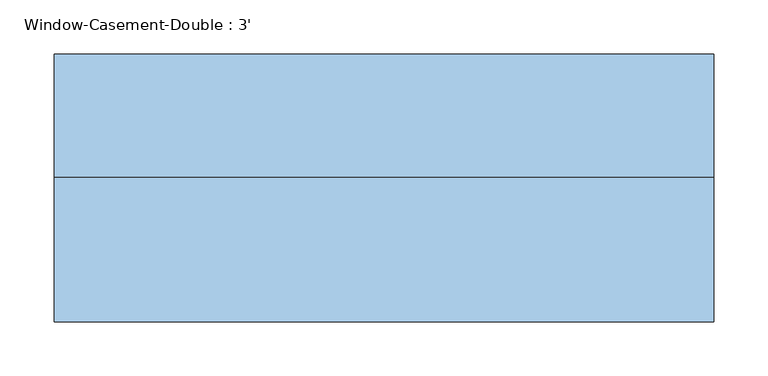
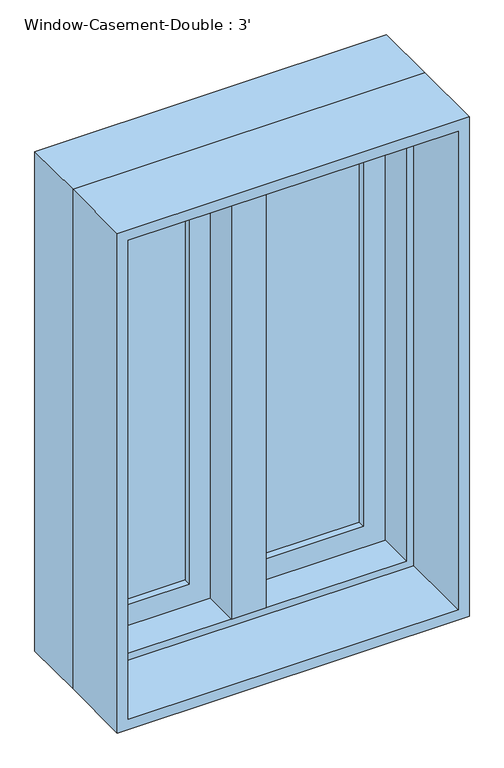
"""IFC4 building model written with IfcOpenShell, lengths in millimetres: window geometry, Window-Casement-Double : 3'."""

from ifc_helpers import new_model, si_unit, frame, origin, place, context, project, spatial, polyline, outline, extrude, faceted_brep, source, transform, mapped, element, save


def window_casement_double_3_c417fced(model_context):
    return source(origin(), model_context, "Body", "SolidModel", [
        faceted_brep([(9.525, 133.35, 1816.1), (-9.525, 133.35, 1816.1), (-9.525, 82.55, 1816.1), (9.525, 82.55, 1816.1), (9.525, 133.35, 927.1), (9.525, 82.55, 927.1), (-9.525, 82.55, 927.1), (-9.525, 133.35, 927.1), (-9.525, 82.55, 946.15), (-9.525, 82.55, 1797.05), (-30.1625, 82.55, 946.15), (-30.1625, 82.55, 1797.05), (-30.1625, 19.05, 946.15), (-30.1625, 19.05, 1797.05), (30.1625, 19.05, 946.15), (30.1625, 19.05, 1797.05), (30.1625, 82.55, 946.15), (30.1625, 82.55, 1797.05), (9.525, 82.55, 946.15), (9.525, 82.55, 1797.05)], [[[0, 1, 2, 3]], [[4, 5, 6, 7]], [[1, 0, 4, 7]], [[2, 1, 7, 6, 8, 9]], [[9, 8, 10, 11]], [[11, 10, 12, 13]], [[13, 12, 14, 15]], [[15, 14, 16, 17]], [[17, 16, 18, 19]], [[0, 3, 19, 18, 5, 4]], [[18, 8, 6, 5]], [[9, 19, 3, 2]], [[8, 18, 16, 14, 12, 10]], [[19, 9, 11, 13, 15, 17]]]),
        extrude(outline(polyline([(-66.675, 114.3), (-66.675, 107.95), (-234.95, 107.95), (-234.95, 114.3), (-66.675, 114.3)])), frame((0.0, 0.0, 984.25), z_axis=(0.0, 0.0, 1.0), x_axis=(1.0, 0.0, 0.0)), (0.0, 0.0, 1.0), 774.7),
        extrude(outline(polyline([(-234.95, 95.25), (-234.95, 101.6), (-66.675, 101.6), (-66.675, 95.25), (-234.95, 95.25)])), frame((0.0, 0.0, 984.25), z_axis=(0.0, 0.0, 1.0), x_axis=(1.0, 0.0, 0.0)), (0.0, 0.0, 1.0), 774.7),
        extrude(outline(polyline([(234.95, 114.3), (234.95, 107.95), (66.675, 107.95), (66.675, 114.3), (234.95, 114.3)])), frame((0.0, 0.0, 984.25), z_axis=(0.0, 0.0, 1.0), x_axis=(1.0, 0.0, 0.0)), (0.0, 0.0, 1.0), 774.7),
        extrude(outline(polyline([(66.675, 95.25), (66.675, 101.6), (234.95, 101.6), (234.95, 95.25), (66.675, 95.25)])), frame((0.0, 0.0, 984.25), z_axis=(0.0, 0.0, 1.0), x_axis=(1.0, 0.0, 0.0)), (0.0, 0.0, 1.0), 774.7),
        extrude(outline(polyline([(1816.1, -292.1), (927.1, -292.1), (927.1, -9.525), (1816.1, -9.525), (1816.1, -292.1)]), holes=[polyline([(1758.95, -66.675), (984.25, -66.675), (984.25, -234.95), (1758.95, -234.95), (1758.95, -66.675)])]), frame((0.0, 82.55, 0.0), z_axis=(0.0, 1.0, 0.0), x_axis=(0.0, 0.0, 1.0)), (0.0, 0.0, 1.0), 44.45),
        extrude(outline(polyline([(927.1, 292.1), (1816.1, 292.1), (1816.1, 9.525), (927.1, 9.525), (927.1, 292.1)]), holes=[polyline([(984.25, 66.675), (1758.95, 66.675), (1758.95, 234.95), (984.25, 234.95), (984.25, 66.675)])]), frame((0.0, 82.55, 0.0), z_axis=(0.0, 1.0, 0.0), x_axis=(0.0, 0.0, 1.0)), (0.0, 0.0, 1.0), 44.45),
        extrude(outline(polyline([(1828.8, -304.8), (914.4, -304.8), (914.4, 304.8), (1828.8, 304.8), (1828.8, -304.8)]), holes=[polyline([(1809.75, 285.75), (933.45, 285.75), (933.45, -285.75), (1809.75, -285.75), (1809.75, 285.75)])]), frame((0.0, -114.3, 0.0), z_axis=(0.0, 1.0, 0.0), x_axis=(0.0, 0.0, 1.0)), (0.0, 0.0, 1.0), 133.35),
        faceted_brep([(273.05, 82.55, 1797.05), (273.05, 19.05, 1797.05), (-273.05, 19.05, 1797.05), (-273.05, 82.55, 1797.05), (292.1, 133.35, 1816.1), (292.1, 82.55, 1816.1), (-292.1, 82.55, 1816.1), (-292.1, 133.35, 1816.1), (304.8, 19.05, 1828.8), (304.8, 133.35, 1828.8), (-304.8, 133.35, 1828.8), (-304.8, 19.05, 1828.8), (-273.05, 19.05, 946.15), (-273.05, 82.55, 946.15), (-292.1, 82.55, 927.1), (-292.1, 133.35, 927.1), (-304.8, 133.35, 914.4), (-304.8, 19.05, 914.4), (273.05, 19.05, 946.15), (273.05, 82.55, 946.15), (292.1, 82.55, 927.1), (292.1, 133.35, 927.1), (304.8, 133.35, 914.4), (304.8, 19.05, 914.4)], [[[0, 1, 2, 3]], [[4, 5, 6, 7]], [[8, 9, 10, 11]], [[3, 2, 12, 13]], [[7, 6, 14, 15]], [[11, 10, 16, 17]], [[13, 12, 18, 19]], [[15, 14, 20, 21]], [[17, 16, 22, 23]], [[11, 17, 23, 8], [1, 18, 12, 2]], [[19, 18, 1, 0]], [[5, 20, 14, 6], [3, 13, 19, 0]], [[21, 20, 5, 4]], [[23, 22, 9, 8]], [[9, 22, 16, 10], [7, 15, 21, 4]]]),
    ])


if __name__ == "__main__":
    model = new_model("IFC4")
    model_context = context("Model", 3, world=origin())
    ifc_project = project(units=[si_unit("LENGTHUNIT", "METRE", prefix="MILLI")], contexts=[model_context])
    site = spatial("IfcSite", under=ifc_project)
    building = spatial("IfcBuilding", under=site)
    placement = place(None, origin())
    window_casement_double_3_shape = window_casement_double_3_c417fced(model_context)
    element("IfcWindow", 1, ObjectType="Window-Casement-Double : 3'", at=placement, inside=building, context=model_context, shape_type="MappedRepresentation", body=[
        mapped(window_casement_double_3_shape, transform((0.0, 0.0, 0.0), x_axis=(1.0, 0.0, 0.0), y_axis=(0.0, 1.0, 0.0), z_axis=(0.0, 0.0, 1.0))),
    ])
    save(model, "model.ifc")

# Revit data of these elements
# Type "Window-Casement-Double : 3'"
#   Type Mark = "19"
#   Fire Rating = "0.5h"
#   Assembly Code = "B2020100"
#   Analytic Construction = "Double glazing - domestic"
#   Frame Extension [instance default] = 0' - 0 1/4"
#   Window Inset [instance default] = 0' - 0"
#   Wall Thickness [instance default] = 0' - 6"
#   Interior Wall Closure [instance default] = 0' - 2 1/4"
#   Half Width = 1' - 0"
#   Visual Light Transmittance = 0.81
#   Thermal Resistance (R) = 1.8146 (h·ft²·°F)/BTU
#   Solar Heat Gain Coefficient = 0.76
#   Rough Width = 2' - 0 1/2"
#   Rough Height = 3' - 0 1/2"
#   Height = 3' - 0"
#   Heat Transfer Coefficient (U) = 0.5511 BTU/(h·ft²·°F)
#   Exterior Wall Closure [instance default] = 0' - 1 1/4"
#   Extension Jamb [instance default] = 0' - 2 1/4"
#   Default Sill Height = 3' - 0"
#   Width = 2' - 0"
#   Muntin Visibility = yes
#   Interior Trim Visibility [instance default] = yes
#   Exterior Trim Visibility [instance default] = yes
#   Extension Jamb Visibility [instance default] = yes
#   Interior Trim Material = Wood - Stained
#   Muntin Pattern = Muntin Pattern_2x2 : Muntin Pattern_2x2
#   Interior Trim = Trim-Window-Interior-Flat : Picture Frame
#   Interior Frame Material = Wood - Stained
#   Glass Panel Material = Glass
#   Exterior Trim Material = Clad - White
#   Exterior Trim = Trim-Window-Exterior-Flat : with Sill
#   Exterior Frame Material = Clad - White
#   Wall Closure = (empty or 0)
# Element 1 (IfcWindow, "Window-Casement-Double : 3'")
#   Wall Thickness = 0' - 9"
#   Extension Jamb = 0' - 5 1/4"
#   Materials on its faces: "Wood - Stained", "Glass", "Clad - White"
# Materials
#   "Wood - Stained": class "Wood", colour RGB 224 178 126, transparency 0, Cost = 0
#   "Glass": class "Glass", colour RGB 0 128 192, transparency 0.75, Description = "Soda Lime Glass", Cost = 0
#   "Clad - White": class "Wood", colour RGB 242 242 238, transparency 0, Cost = 0
